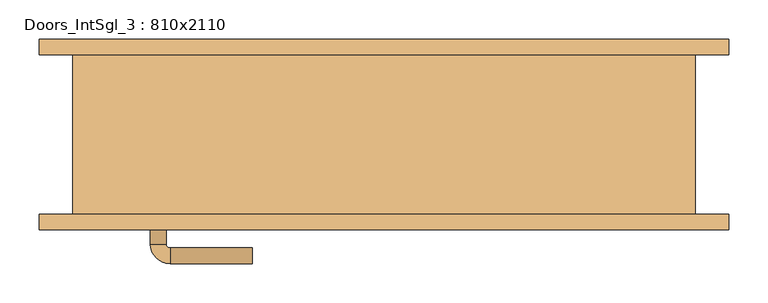
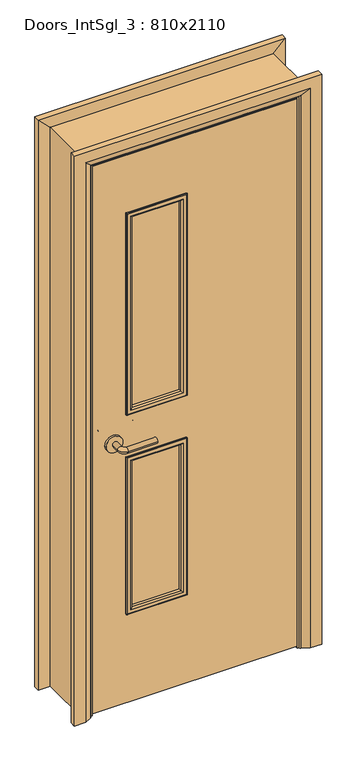
"""IFC4 building model written with IfcOpenShell, lengths in millimetres: door geometry, Doors_IntSgl_3 : 810x2110."""

from ifc_helpers import new_model, si_unit, point, frame, frame_2d, origin, place, context, project, spatial, polyline, circle_curve, ellipse_curve, trimmed, segment, composite_curve, outline, extrude, faceted_brep, source, transform, mapped, element, save
from ifc_brep_helpers import plane_surface, cylinder_surface, revolved_surface, advanced_brep


def doors_intsgl_3_810x2110_fc3e9706(model_context):
    return source(origin(), model_context, "Body", "SolidModel", [
        advanced_brep(
        [(-298.0, -55.6, 1000.0), (-278.0, -55.6, 1000.0), (-298.0, -25.6, 1000.0), (-278.0, -25.6, 1000.0), (-273.0, -20.6, 1000.0), (-273.0, -0.6, 1000.0), (-168.0, -0.6, 1000.0), (-168.0, -20.6, 1000.0)],
        [
            (0, 1, circle_curve(frame((-288.0, -55.6, 1000.0), z_axis=(0.0, -1.0, 0.0), x_axis=(1.0, 0.0, 0.0)), 10.0)),
            (1, 0, circle_curve(frame((-288.0, -55.6, 1000.0), z_axis=(0.0, -1.0, 0.0), x_axis=(1.0, 0.0, 0.0)), 10.0)),
            (0, 2),
            (2, 3, circle_curve(frame((-288.0, -25.6, 1000.0), z_axis=(0.0, -1.0, 0.0), x_axis=(1.0, 0.0, 0.0)), 10.0)),
            (3, 1),
            (3, 2, circle_curve(frame((-288.0, -25.6, 1000.0), z_axis=(0.0, -1.0, 0.0), x_axis=(1.0, 0.0, 0.0)), 10.0)),
            (4, 3, circle_curve(frame((-273.0, -25.6, 1000.0), z_axis=(0.0, 0.0, 1.0), x_axis=(-1.0, 0.0, 0.0)), 5.0)),
            (2, 5, circle_curve(frame((-273.0, -25.6, 1000.0), z_axis=(0.0, 0.0, -1.0), x_axis=(-1.0, 0.0, 0.0)), 25.0)),
            (5, 4, circle_curve(frame((-273.0, -10.6, 1000.0), z_axis=(-1.0, 0.0, 0.0), x_axis=(0.0, -1.0, 0.0)), 10.0)),
            (4, 5, circle_curve(frame((-273.0, -10.6, 1000.0), z_axis=(-1.0, 0.0, 0.0), x_axis=(0.0, -1.0, 0.0)), 10.0)),
            (6, 7, circle_curve(frame((-168.0, -10.6, 1000.0), z_axis=(1.0, 0.0, 0.0), x_axis=(0.0, -1.0, 0.0)), 10.0)),
            (7, 6, circle_curve(frame((-168.0, -10.6, 1000.0), z_axis=(1.0, 0.0, 0.0), x_axis=(0.0, -1.0, 0.0)), 10.0)),
            (5, 6),
            (7, 4),
        ],
        [
            plane_surface(frame((-288.0, -55.6, 1000.0), z_axis=(0.0, -1.0, 0.0), x_axis=(0.0, 0.0, 1.0))),
            cylinder_surface(frame((-288.0, -55.6, 1000.0), z_axis=(0.0, -1.0, 0.0), x_axis=(1.0, 0.0, 0.0)), 10.0),
            revolved_surface(trimmed(ellipse_curve(frame((-288.0, -25.6, 1000.0), z_axis=(0.0, -1.0, 0.0), x_axis=(1.0, 0.0, 0.0)), 10.0, 10.0), [point((-298.0, -25.6, 1000.0))], [point((-278.0, -25.6, 1000.0))], True, "CARTESIAN"), (-273.0, -25.6, 1000.0), (0.0, 0.0, -1.0)),
            revolved_surface(trimmed(ellipse_curve(frame((-288.0, -25.6, 1000.0), z_axis=(0.0, -1.0, 0.0), x_axis=(1.0, 0.0, 0.0)), 10.0, 10.0), [point((-278.0, -25.6, 1000.0))], [point((-298.0, -25.6, 1000.0))], True, "CARTESIAN"), (-273.0, -25.6, 1000.0), (0.0, 0.0, -1.0)),
            plane_surface(frame((-168.0, -10.6, 1000.0), z_axis=(1.0, 0.0, 0.0), x_axis=(0.0, 0.0, 1.0))),
            cylinder_surface(frame((-273.0, -10.6, 1000.0), z_axis=(-1.0, 0.0, 0.0), x_axis=(0.0, -1.0, 0.0)), 10.0),
        ],
        [
            (0, [[1, 2]]),
            (1, [[-1, 3, 4, 5]]),
            (1, [[-2, -5, 6, -3]]),
            (2, [[7, -4, 8, 9]]),
            (3, [[-8, -6, -7, 10]]),
            (4, [[11, 12]]),
            (5, [[-9, 13, -12, 14]]),
            (5, [[-10, -14, -11, -13]]),
        ],
    ),
        extrude(outline(composite_curve([segment(trimmed(circle_curve(frame_2d((1000.0, -290.5)), 30.0), [point((1000.0, -320.5))], [point((1000.0, -260.5))], False, "CARTESIAN"), True, "CONTINUOUS"), segment(trimmed(circle_curve(frame_2d((1000.0, -290.5)), 30.0), [point((1000.0, -260.5))], [point((1000.0, -320.5))], False, "CARTESIAN"), True, "CONTINUOUS")], self_intersect=False)), frame((0.0, -63.6, 0.0), z_axis=(0.0, 1.0, 0.0), x_axis=(0.0, 0.0, 1.0)), (0.0, 0.0, 1.0), 8.0),
        advanced_brep(
        [(-298.0, -109.6, 1000.0), (-278.0, -109.6, 1000.0), (-278.0, -139.6, 1000.0), (-298.0, -139.6, 1000.0), (-273.0, -144.6, 1000.0), (-273.0, -164.6, 1000.0), (-168.0, -164.6, 1000.0), (-168.0, -144.6, 1000.0)],
        [
            (0, 1, circle_curve(frame((-288.0, -109.6, 1000.0), z_axis=(0.0, 1.0, 0.0), x_axis=(1.0, 0.0, 0.0)), 10.0)),
            (1, 0, circle_curve(frame((-288.0, -109.6, 1000.0), z_axis=(0.0, 1.0, 0.0), x_axis=(1.0, 0.0, 0.0)), 10.0)),
            (1, 2),
            (2, 3, circle_curve(frame((-288.0, -139.6, 1000.0), z_axis=(0.0, 1.0, 0.0), x_axis=(1.0, 0.0, 0.0)), 10.0)),
            (3, 0),
            (3, 2, circle_curve(frame((-288.0, -139.6, 1000.0), z_axis=(0.0, 1.0, 0.0), x_axis=(1.0, 0.0, 0.0)), 10.0)),
            (4, 5, circle_curve(frame((-273.0, -154.6, 1000.0), z_axis=(-1.0, 0.0, 0.0), x_axis=(0.0, 1.0, 0.0)), 10.0)),
            (5, 3, circle_curve(frame((-273.0, -139.6, 1000.0), z_axis=(0.0, 0.0, -1.0), x_axis=(-1.0, 0.0, 0.0)), 25.0)),
            (2, 4, circle_curve(frame((-273.0, -139.6, 1000.0), z_axis=(0.0, 0.0, 1.0), x_axis=(-1.0, 0.0, 0.0)), 5.0)),
            (5, 4, circle_curve(frame((-273.0, -154.6, 1000.0), z_axis=(-1.0, 0.0, 0.0), x_axis=(0.0, 1.0, 0.0)), 10.0)),
            (6, 7, circle_curve(frame((-168.0, -154.6, 1000.0), z_axis=(1.0, 0.0, 0.0), x_axis=(0.0, 1.0, 0.0)), 10.0)),
            (7, 6, circle_curve(frame((-168.0, -154.6, 1000.0), z_axis=(1.0, 0.0, 0.0), x_axis=(0.0, 1.0, 0.0)), 10.0)),
            (4, 7),
            (6, 5),
        ],
        [
            plane_surface(frame((-288.0, -109.6, 1000.0), z_axis=(0.0, 1.0, 0.0), x_axis=(0.0, 0.0, 1.0))),
            cylinder_surface(frame((-288.0, -109.6, 1000.0), z_axis=(0.0, 1.0, 0.0), x_axis=(1.0, 0.0, 0.0)), 10.0),
            revolved_surface(trimmed(ellipse_curve(frame((-288.0, -139.6, 1000.0), z_axis=(0.0, -1.0, 0.0), x_axis=(1.0, 0.0, 0.0)), 10.0, 10.0), [point((-298.0, -139.6, 1000.0))], [point((-278.0, -139.6, 1000.0))], True, "CARTESIAN"), (-273.0, -139.6, 1000.0), (0.0, 0.0, -1.0)),
            revolved_surface(trimmed(ellipse_curve(frame((-288.0, -139.6, 1000.0), z_axis=(0.0, -1.0, 0.0), x_axis=(1.0, 0.0, 0.0)), 10.0, 10.0), [point((-278.0, -139.6, 1000.0))], [point((-298.0, -139.6, 1000.0))], True, "CARTESIAN"), (-273.0, -139.6, 1000.0), (0.0, 0.0, -1.0)),
            plane_surface(frame((-168.0, -154.6, 1000.0), z_axis=(1.0, 0.0, 0.0), x_axis=(0.0, 0.0, 1.0))),
            cylinder_surface(frame((-273.0, -154.6, 1000.0), z_axis=(-1.0, 0.0, 0.0), x_axis=(0.0, 1.0, 0.0)), 10.0),
        ],
        [
            (0, [[1, 2]]),
            (1, [[3, 4, 5, -2]]),
            (1, [[-5, 6, -3, -1]]),
            (2, [[7, 8, -4, 9]]),
            (3, [[10, -9, -6, -8]]),
            (4, [[11, 12]]),
            (5, [[13, -11, 14, -7]]),
            (5, [[-14, -12, -13, -10]]),
        ],
    ),
        extrude(outline(composite_curve([segment(trimmed(circle_curve(frame_2d((1000.0, -290.5)), 30.0), [point((1000.0, -320.5))], [point((1000.0, -260.5))], False, "CARTESIAN"), True, "CONTINUOUS"), segment(trimmed(circle_curve(frame_2d((1000.0, -290.5)), 30.0), [point((1000.0, -260.5))], [point((1000.0, -320.5))], False, "CARTESIAN"), True, "CONTINUOUS")], self_intersect=False)), frame((0.0, -109.6, 0.0), z_axis=(0.0, 1.0, 0.0), x_axis=(0.0, 0.0, 1.0)), (0.0, 0.0, 1.0), 8.0),
        extrude(outline(polyline([(2068.0, -363.0), (8.0, -363.0), (8.0, 363.0), (2068.0, 363.0), (2068.0, -363.0)]), holes=[polyline([(1843.0, -38.0), (1100.0, -38.0), (1100.0, -238.0), (1843.0, -238.0), (1843.0, -38.0)]), polyline([(925.0, -238.0), (925.0, -38.0), (350.0, -38.0), (350.0, -238.0), (925.0, -238.0)])]), frame((0.0, -101.6, 0.0), z_axis=(0.0, 1.0, 0.0), x_axis=(0.0, 0.0, 1.0)), (0.0, 0.0, 1.0), 38.0),
        faceted_brep([(-365.0, -101.6, 0.0), (-397.0, -101.6, 0.0), (-397.0, 101.6, 0.0), (-365.0, 101.6, 0.0), (-365.0, 101.6, 2070.0), (-365.0, -101.6, 2070.0), (-397.0, 101.6, 2102.0), (-397.0, -101.6, 2102.0), (365.0, -101.6, 0.0), (365.0, 101.6, 0.0), (397.0, 101.6, 0.0), (397.0, -101.6, 0.0), (365.0, -101.6, 2070.0), (397.0, -101.6, 2102.0), (397.0, 101.6, 2102.0), (365.0, 101.6, 2070.0)], [[[0, 1, 2, 3]], [[3, 4, 5, 0]], [[2, 6, 4, 3]], [[1, 7, 6, 2]], [[0, 5, 7, 1]], [[8, 9, 10, 11]], [[12, 8, 11, 13]], [[13, 11, 10, 14]], [[14, 10, 9, 15]], [[15, 9, 8, 12]], [[4, 15, 12, 5]], [[6, 14, 15, 4]], [[7, 13, 14, 6]], [[5, 12, 13, 7]]]),
        advanced_brep(
        [(-440.0, 121.6, 0.0), (-400.0, 121.6, 0.0), (-374.0, 107.6, 0.0), (-370.0, 101.6, 0.0), (-440.0, 101.6, 0.0), (-440.0, 101.6, 2145.0), (-440.0, 121.6, 2145.0), (-370.0, 101.6, 2075.0), (-374.0, 107.6, 2079.0), (-400.0, 121.6, 2105.0), (440.0, 121.6, 0.0), (440.0, 101.6, 0.0), (370.0, 101.6, 0.0), (374.0, 107.6, 0.0), (400.0, 121.6, 0.0), (440.0, 121.6, 2145.0), (400.0, 121.6, 2105.0), (374.0, 107.6, 2079.0), (370.0, 101.6, 2075.0), (440.0, 101.6, 2145.0)],
        [
            (0, 1),
            (1, 2),
            (2, 3, circle_curve(frame((-378.0, 100.6, 0.0), z_axis=(0.0, 0.0, -1.0), x_axis=(-1.0, 0.0, 0.0)), 8.0622577)),
            (3, 4),
            (4, 0),
            (4, 5),
            (5, 6),
            (6, 0),
            (3, 7),
            (7, 5),
            (2, 8),
            (8, 7, ellipse_curve(frame((-378.0, 100.6, 2083.0), z_axis=(-0.7071067811865475, 0.0, -0.7071067811865475), x_axis=(0.7071067811865474, 0.0, -0.7071067811865476)), 11.4017543, 8.0622577)),
            (1, 9),
            (9, 8),
            (6, 9),
            (10, 11),
            (11, 12),
            (12, 13, circle_curve(frame((378.0, 100.6, 0.0), z_axis=(0.0, 0.0, -1.0), x_axis=(1.0, 0.0, 0.0)), 8.0622577)),
            (13, 14),
            (14, 10),
            (15, 10),
            (14, 16),
            (16, 15),
            (13, 17),
            (17, 16),
            (12, 18),
            (18, 17, ellipse_curve(frame((378.0, 100.6, 2083.0), z_axis=(0.7071067811865475, 0.0, -0.7071067811865475), x_axis=(0.7071067811865474, 0.0, 0.7071067811865476)), 11.4017543, 8.0622577)),
            (11, 19),
            (19, 18),
            (15, 19),
            (5, 19),
            (15, 6),
            (7, 18),
            (8, 17),
            (9, 16),
        ],
        [
            plane_surface(frame((-370.0, 174.4010989, 0.0), z_axis=(0.0, 0.0, -1.0), x_axis=(1.0, 0.0, 0.0))),
            plane_surface(frame((-440.0, 121.6, 0.0), z_axis=(-1.0, 0.0, 0.0), x_axis=(0.0, 0.0, 1.0))),
            plane_surface(frame((-440.0, 101.6, 0.0), z_axis=(0.0, -1.0, 0.0), x_axis=(0.0, 0.0, 1.0))),
            cylinder_surface(frame((-378.0, 100.6, 0.0), z_axis=(0.0, 0.0, -1.0), x_axis=(-1.0, 0.0, 0.0)), 8.0622577),
            plane_surface(frame((-374.0, 107.6, 0.0), z_axis=(0.4740998230350183, 0.8804710999221749, 0.0), x_axis=(0.0, 0.0, 1.0))),
            plane_surface(frame((-400.0, 121.6, 0.0), z_axis=(0.0, 1.0, 0.0), x_axis=(0.0, 0.0, 1.0))),
            plane_surface(frame((370.0, 174.4010989, 0.0), z_axis=(0.0, 0.0, -1.0), x_axis=(-1.0, 0.0, 0.0))),
            plane_surface(frame((400.0, 121.6, 2105.0), z_axis=(0.0, 1.0, 0.0), x_axis=(0.0, 0.0, -1.0))),
            plane_surface(frame((374.0, 107.6, 2079.0), z_axis=(-0.4740998230350183, 0.8804710999221749, 0.0), x_axis=(0.0, 0.0, -1.0))),
            cylinder_surface(frame((378.0, 100.6, 2075.0), z_axis=(0.0, 0.0, 1.0), x_axis=(1.0, 0.0, 0.0)), 8.0622577),
            plane_surface(frame((440.0, 101.6, 2145.0), z_axis=(0.0, -1.0, 0.0), x_axis=(0.0, 0.0, -1.0))),
            plane_surface(frame((440.0, 121.6, 2145.0), z_axis=(1.0, 0.0, 0.0), x_axis=(0.0, 0.0, -1.0))),
            plane_surface(frame((-440.0, 121.6, 2145.0), z_axis=(0.0, 0.0, 1.0), x_axis=(1.0, 0.0, 0.0))),
            plane_surface(frame((-440.0, 101.6, 2145.0), z_axis=(0.0, -1.0, 0.0), x_axis=(1.0, 0.0, 0.0))),
            cylinder_surface(frame((-370.0, 100.6, 2083.0), z_axis=(-1.0, 0.0, 0.0), x_axis=(0.0, 0.0, 1.0)), 8.0622577),
            plane_surface(frame((-374.0, 107.6, 2079.0), z_axis=(0.0, 0.8804710999221749, -0.4740998230350183), x_axis=(1.0, 0.0, 0.0))),
            plane_surface(frame((-400.0, 121.6, 2105.0), z_axis=(0.0, 1.0, 0.0), x_axis=(1.0, 0.0, 0.0))),
        ],
        [
            (0, [[1, 2, 3, 4, 5]]),
            (1, [[6, 7, 8, -5]]),
            (2, [[9, 10, -6, -4]]),
            (3, [[11, 12, -9, -3]]),
            (4, [[13, 14, -11, -2]]),
            (5, [[-8, 15, -13, -1]]),
            (6, [[16, 17, 18, 19, 20]]),
            (7, [[21, -20, 22, 23]]),
            (8, [[-22, -19, 24, 25]]),
            (9, [[-24, -18, 26, 27]]),
            (10, [[-26, -17, 28, 29]]),
            (11, [[-28, -16, -21, 30]]),
            (12, [[31, -30, 32, -7]]),
            (13, [[33, -29, -31, -10]]),
            (14, [[34, -27, -33, -12]]),
            (15, [[35, -25, -34, -14]]),
            (16, [[-32, -23, -35, -15]]),
        ],
    ),
        extrude(outline(polyline([(0.0, -346.0), (2051.0, -346.0), (2051.0, 346.0), (0.0, 346.0), (0.0, 365.0), (2070.0, 365.0), (2070.0, -365.0), (0.0, -365.0), (0.0, -346.0)])), frame((0.0, -61.6, 0.0), z_axis=(0.0, 1.0, 0.0), x_axis=(0.0, 0.0, 1.0)), (0.0, 0.0, 1.0), 32.0),
        advanced_brep(
        [(440.0, -121.6, 0.0), (400.0, -121.6, 0.0), (374.0, -107.6, 0.0), (370.0, -101.6, 0.0), (440.0, -101.6, 0.0), (440.0, -101.6, 2145.0), (440.0, -121.6, 2145.0), (370.0, -101.6, 2075.0), (-370.0, -101.6, 2075.0), (-370.0, -101.6, 0.0), (-440.0, -101.6, 0.0), (-440.0, -101.6, 2145.0), (374.0, -107.6, 2079.0), (400.0, -121.6, 2105.0), (-440.0, -121.6, 2145.0), (-440.0, -121.6, 0.0), (-400.0, -121.6, 0.0), (-400.0, -121.6, 2105.0), (-374.0, -107.6, 0.0), (-374.0, -107.6, 2079.0)],
        [
            (0, 1),
            (1, 2),
            (2, 3, circle_curve(frame((378.0, -100.6, 0.0), z_axis=(0.0, 0.0, -1.0), x_axis=(1.0, 0.0, 0.0)), 8.0622577)),
            (3, 4),
            (4, 0),
            (4, 5),
            (5, 6),
            (6, 0),
            (3, 7),
            (7, 8),
            (8, 9),
            (9, 10),
            (10, 11),
            (11, 5),
            (2, 12),
            (12, 7, ellipse_curve(frame((378.0, -100.6, 2083.0), z_axis=(0.7071067811865475, 0.0, -0.7071067811865475), x_axis=(-0.7071067811865474, 0.0, -0.7071067811865476)), 11.4017543, 8.0622577)),
            (1, 13),
            (13, 12),
            (6, 14),
            (14, 15),
            (15, 16),
            (16, 17),
            (17, 13),
            (10, 15),
            (14, 11),
            (9, 18, circle_curve(frame((-378.0, -100.6, 0.0), z_axis=(0.0, 0.0, -1.0), x_axis=(-1.0, 0.0, 0.0)), 8.0622577)),
            (18, 16),
            (19, 18),
            (8, 19, ellipse_curve(frame((-378.0, -100.6, 2083.0), z_axis=(-0.7071067811865475, 0.0, -0.7071067811865475), x_axis=(-0.7071067811865474, 0.0, 0.7071067811865476)), 11.4017543, 8.0622577)),
            (19, 17),
            (12, 19),
        ],
        [
            plane_surface(frame((370.0, -101.6, 0.0), z_axis=(0.0, 0.0, -1.0), x_axis=(0.0, 1.0, 0.0))),
            plane_surface(frame((440.0, -121.6, 0.0), z_axis=(1.0, 0.0, 0.0), x_axis=(0.0, 0.0, 1.0))),
            plane_surface(frame((440.0, -101.6, 0.0), z_axis=(0.0, 1.0, 0.0), x_axis=(0.0, 0.0, 1.0))),
            cylinder_surface(frame((378.0, -100.6, 0.0), z_axis=(0.0, 0.0, -1.0), x_axis=(1.0, 0.0, 0.0)), 8.0622577),
            plane_surface(frame((374.0, -107.6, 0.0), z_axis=(-0.4740998230350126, -0.8804710999221779, 0.0), x_axis=(0.0, 0.0, 1.0))),
            plane_surface(frame((400.0, -121.6, 0.0), z_axis=(0.0, -1.0, 0.0), x_axis=(0.0, 0.0, 1.0))),
            plane_surface(frame((-440.0, -121.6, 2145.0), z_axis=(-1.0, 0.0, 0.0), x_axis=(0.0, 0.0, -1.0))),
            plane_surface(frame((-370.0, -101.6, 0.0), z_axis=(0.0, 0.0, -1.0), x_axis=(0.0, 1.0, 0.0))),
            cylinder_surface(frame((-378.0, -100.6, 2075.0), z_axis=(0.0, 0.0, 1.0), x_axis=(-1.0, 0.0, 0.0)), 8.0622577),
            plane_surface(frame((-374.0, -107.6, 2079.0), z_axis=(0.4740998230350183, -0.8804710999221749, 0.0), x_axis=(0.0, 0.0, -1.0))),
            plane_surface(frame((440.0, -121.6, 2145.0), z_axis=(0.0, 0.0, 1.0), x_axis=(-1.0, 0.0, 0.0))),
            cylinder_surface(frame((370.0, -100.6, 2083.0), z_axis=(1.0, 0.0, 0.0), x_axis=(0.0, 0.0, 1.0)), 8.0622577),
            plane_surface(frame((374.0, -107.6, 2079.0), z_axis=(0.0, -0.8804710999221763, -0.4740998230350154), x_axis=(-1.0, 0.0, 0.0))),
        ],
        [
            (0, [[1, 2, 3, 4, 5]]),
            (1, [[6, 7, 8, -5]]),
            (2, [[9, 10, 11, 12, 13, 14, -6, -4]]),
            (3, [[15, 16, -9, -3]]),
            (4, [[17, 18, -15, -2]]),
            (5, [[-8, 19, 20, 21, 22, 23, -17, -1]]),
            (6, [[-13, 24, -20, 25]]),
            (7, [[-24, -12, 26, 27, -21]]),
            (8, [[28, -26, -11, 29]]),
            (9, [[-22, -27, -28, 30]]),
            (10, [[-14, -25, -19, -7]]),
            (11, [[31, -29, -10, -16]]),
            (12, [[-23, -30, -31, -18]]),
        ],
    ),
        advanced_brep(
        [(-30.0, -105.6, 1851.0), (-30.0, -105.6, 1092.0), (-30.0, -101.6, 1092.0), (-30.0, -101.6, 1851.0), (-32.0, -107.6, 1849.0), (-32.0, -107.6, 1094.0), (-50.0, -102.6, 1831.0), (-50.0, -102.6, 1112.0), (-45.0, -107.6, 1107.0), (-45.0, -107.6, 1836.0), (-50.0, -91.6, 1831.0), (-50.0, -91.6, 1112.0), (-38.0, -101.6, 1843.0), (-38.0, -101.6, 1100.0), (-38.0, -91.6, 1100.0), (-38.0, -91.6, 1843.0), (-246.0, -105.6, 1092.0), (-246.0, -101.6, 1092.0), (-244.0, -107.6, 1094.0), (-226.0, -102.6, 1112.0), (-231.0, -107.6, 1107.0), (-226.0, -91.6, 1112.0), (-238.0, -101.6, 1100.0), (-238.0, -91.6, 1100.0), (-246.0, -105.6, 1851.0), (-246.0, -101.6, 1851.0), (-244.0, -107.6, 1849.0), (-226.0, -102.6, 1831.0), (-231.0, -107.6, 1836.0), (-226.0, -91.6, 1831.0), (-238.0, -101.6, 1843.0), (-238.0, -91.6, 1843.0)],
        [
            (0, 1),
            (1, 2),
            (2, 3),
            (3, 0),
            (4, 5),
            (5, 1, ellipse_curve(frame((-32.0, -105.6, 1094.0), z_axis=(0.7071067811865475, 0.0, 0.7071067811865475), x_axis=(-0.7071067811865474, 0.0, 0.7071067811865476)), 2.8284271, 2.0)),
            (0, 4, ellipse_curve(frame((-32.0, -105.6, 1849.0), z_axis=(0.7071067811865475, 0.0, -0.7071067811865475), x_axis=(0.7071067811865474, 0.0, 0.7071067811865476)), 2.8284271, 2.0)),
            (6, 7),
            (7, 8, ellipse_curve(frame((-45.0, -102.6, 1107.0), z_axis=(0.7071067811865475, 0.0, 0.7071067811865475), x_axis=(-0.7071067811865474, 0.0, 0.7071067811865476)), 7.0710678, 5.0)),
            (8, 9),
            (9, 6, ellipse_curve(frame((-45.0, -102.6, 1836.0), z_axis=(0.7071067811865475, 0.0, -0.7071067811865475), x_axis=(0.7071067811865474, 0.0, 0.7071067811865476)), 7.0710678, 5.0)),
            (10, 11),
            (11, 7),
            (6, 10),
            (12, 13),
            (13, 14),
            (14, 15),
            (15, 12),
            (1, 16),
            (16, 17),
            (17, 2),
            (5, 18),
            (18, 16, ellipse_curve(frame((-244.0, -105.6, 1094.0), z_axis=(0.7071067811865475, 0.0, -0.7071067811865475), x_axis=(0.7071067811865476, 0.0, 0.7071067811865474)), 2.8284271, 2.0)),
            (7, 19),
            (19, 20, ellipse_curve(frame((-231.0, -102.6, 1107.0), z_axis=(0.7071067811865475, 0.0, -0.7071067811865475), x_axis=(0.7071067811865476, 0.0, 0.7071067811865474)), 7.0710678, 5.0)),
            (20, 8),
            (11, 21),
            (21, 19),
            (13, 22),
            (22, 23),
            (23, 14),
            (16, 24),
            (24, 25),
            (25, 17),
            (18, 26),
            (26, 24, ellipse_curve(frame((-244.0, -105.6, 1849.0), z_axis=(-0.7071067811865475, 0.0, -0.7071067811865475), x_axis=(0.7071067811865474, 0.0, -0.7071067811865476)), 2.8284271, 2.0)),
            (19, 27),
            (27, 28, ellipse_curve(frame((-231.0, -102.6, 1836.0), z_axis=(-0.7071067811865475, 0.0, -0.7071067811865475), x_axis=(0.7071067811865474, 0.0, -0.7071067811865476)), 7.0710678, 5.0)),
            (28, 20),
            (21, 29),
            (29, 27),
            (22, 30),
            (30, 31),
            (31, 23),
            (24, 0),
            (3, 25),
            (26, 4),
            (28, 9),
            (27, 6),
            (29, 10),
            (31, 15),
            (30, 12),
        ],
        [
            plane_surface(frame((-30.0, -101.6, 1851.0), z_axis=(1.0, 0.0, 0.0), x_axis=(0.0, 0.0, -1.0))),
            cylinder_surface(frame((-32.0, -105.6, 1843.0), z_axis=(0.0, 0.0, 1.0), x_axis=(1.0, 0.0, 0.0)), 2.0),
            cylinder_surface(frame((-45.0, -102.6, 1843.0), z_axis=(0.0, 0.0, 1.0), x_axis=(1.0, 0.0, 0.0)), 5.0),
            plane_surface(frame((-50.0, -102.6, 1831.0), z_axis=(-1.0, 0.0, 0.0), x_axis=(0.0, 0.0, -1.0))),
            plane_surface(frame((-38.0, -91.6, 1843.0), z_axis=(1.0, 0.0, 0.0), x_axis=(0.0, 0.0, -1.0))),
            plane_surface(frame((-30.0, -101.6, 1092.0), z_axis=(0.0, 0.0, -1.0), x_axis=(-1.0, 0.0, 0.0))),
            cylinder_surface(frame((-38.0, -105.6, 1094.0), z_axis=(1.0, 0.0, 0.0), x_axis=(0.0, 0.0, -1.0)), 2.0),
            cylinder_surface(frame((-38.0, -102.6, 1107.0), z_axis=(1.0, 0.0, 0.0), x_axis=(0.0, 0.0, -1.0)), 5.0),
            plane_surface(frame((-50.0, -102.6, 1112.0), z_axis=(0.0, 0.0, 1.0), x_axis=(-1.0, 0.0, 0.0))),
            plane_surface(frame((-38.0, -91.6, 1100.0), z_axis=(0.0, 0.0, -1.0), x_axis=(-1.0, 0.0, 0.0))),
            plane_surface(frame((-246.0, -101.6, 1092.0), z_axis=(-1.0, 0.0, 0.0), x_axis=(0.0, 0.0, 1.0))),
            cylinder_surface(frame((-244.0, -105.6, 1100.0), z_axis=(0.0, 0.0, -1.0), x_axis=(-1.0, 0.0, 0.0)), 2.0),
            cylinder_surface(frame((-231.0, -102.6, 1100.0), z_axis=(0.0, 0.0, -1.0), x_axis=(-1.0, 0.0, 0.0)), 5.0),
            plane_surface(frame((-226.0, -102.6, 1112.0), z_axis=(1.0, 0.0, 0.0), x_axis=(0.0, 0.0, 1.0))),
            plane_surface(frame((-238.0, -91.6, 1100.0), z_axis=(-1.0, 0.0, 0.0), x_axis=(0.0, 0.0, 1.0))),
            plane_surface(frame((-246.0, -101.6, 1851.0), z_axis=(0.0, 0.0, 1.0), x_axis=(1.0, 0.0, 0.0))),
            cylinder_surface(frame((-238.0, -105.6, 1849.0), z_axis=(-1.0, 0.0, 0.0), x_axis=(0.0, 0.0, 1.0)), 2.0),
            plane_surface(frame((-244.0, -107.6, 1849.0), z_axis=(0.0, -1.0, 0.0), x_axis=(1.0, 0.0, 0.0))),
            cylinder_surface(frame((-238.0, -102.6, 1836.0), z_axis=(-1.0, 0.0, 0.0), x_axis=(0.0, 0.0, 1.0)), 5.0),
            plane_surface(frame((-226.0, -102.6, 1831.0), z_axis=(0.0, 0.0, -1.0), x_axis=(1.0, 0.0, 0.0))),
            plane_surface(frame((-226.0, -91.6, 1831.0), z_axis=(0.0, 1.0, 0.0), x_axis=(1.0, 0.0, 0.0))),
            plane_surface(frame((-238.0, -91.6, 1843.0), z_axis=(0.0, 0.0, 1.0), x_axis=(1.0, 0.0, 0.0))),
            plane_surface(frame((-238.0, -101.6, 1843.0), z_axis=(0.0, 1.0, 0.0), x_axis=(1.0, 0.0, 0.0))),
        ],
        [
            (0, [[1, 2, 3, 4]]),
            (1, [[5, 6, -1, 7]]),
            (2, [[8, 9, 10, 11]]),
            (3, [[12, 13, -8, 14]]),
            (4, [[15, 16, 17, 18]]),
            (5, [[19, 20, 21, -2]]),
            (6, [[22, 23, -19, -6]]),
            (7, [[24, 25, 26, -9]]),
            (8, [[27, 28, -24, -13]]),
            (9, [[29, 30, 31, -16]]),
            (10, [[32, 33, 34, -20]]),
            (11, [[35, 36, -32, -23]]),
            (12, [[37, 38, 39, -25]]),
            (13, [[40, 41, -37, -28]]),
            (14, [[42, 43, 44, -30]]),
            (15, [[45, -4, 46, -33]]),
            (16, [[47, -7, -45, -36]]),
            (17, [[-5, -47, -35, -22], [-10, -26, -39, 48]]),
            (18, [[49, -11, -48, -38]]),
            (19, [[50, -14, -49, -41]]),
            (20, [[-17, -31, -44, 51], [-12, -50, -40, -27]]),
            (21, [[52, -18, -51, -43]]),
            (22, [[-3, -21, -34, -46], [-15, -52, -42, -29]]),
        ],
    ),
        advanced_brep(
        [(-38.0, -73.6, 1843.0), (-38.0, -73.6, 1100.0), (-38.0, -63.6, 1100.0), (-38.0, -63.6, 1843.0), (-50.0, -62.6, 1831.0), (-50.0, -62.6, 1112.0), (-50.0, -73.6, 1112.0), (-50.0, -73.6, 1831.0), (-45.0, -57.6, 1836.0), (-45.0, -57.6, 1107.0), (-30.0, -59.6, 1851.0), (-30.0, -59.6, 1092.0), (-32.0, -57.6, 1094.0), (-32.0, -57.6, 1849.0), (-30.0, -63.6, 1851.0), (-30.0, -63.6, 1092.0), (-238.0, -73.6, 1100.0), (-238.0, -63.6, 1100.0), (-226.0, -62.6, 1112.0), (-226.0, -73.6, 1112.0), (-231.0, -57.6, 1107.0), (-246.0, -59.6, 1092.0), (-244.0, -57.6, 1094.0), (-246.0, -63.6, 1092.0), (-238.0, -73.6, 1843.0), (-238.0, -63.6, 1843.0), (-226.0, -62.6, 1831.0), (-226.0, -73.6, 1831.0), (-231.0, -57.6, 1836.0), (-246.0, -59.6, 1851.0), (-244.0, -57.6, 1849.0), (-246.0, -63.6, 1851.0)],
        [
            (0, 1),
            (1, 2),
            (2, 3),
            (3, 0),
            (4, 5),
            (5, 6),
            (6, 7),
            (7, 4),
            (8, 9),
            (9, 5, ellipse_curve(frame((-45.0, -62.6, 1107.0), z_axis=(0.7071067811865475, 0.0, 0.7071067811865475), x_axis=(-0.7071067811865474, 0.0, 0.7071067811865476)), 7.0710678, 5.0)),
            (4, 8, ellipse_curve(frame((-45.0, -62.6, 1836.0), z_axis=(0.7071067811865475, 0.0, -0.7071067811865475), x_axis=(0.7071067811865474, 0.0, 0.7071067811865476)), 7.0710678, 5.0)),
            (10, 11),
            (11, 12, ellipse_curve(frame((-32.0, -59.6, 1094.0), z_axis=(0.7071067811865475, 0.0, 0.7071067811865475), x_axis=(-0.7071067811865474, 0.0, 0.7071067811865476)), 2.8284271, 2.0)),
            (12, 13),
            (13, 10, ellipse_curve(frame((-32.0, -59.6, 1849.0), z_axis=(0.7071067811865475, 0.0, -0.7071067811865475), x_axis=(0.7071067811865474, 0.0, 0.7071067811865476)), 2.8284271, 2.0)),
            (14, 15),
            (15, 11),
            (10, 14),
            (1, 16),
            (16, 17),
            (17, 2),
            (5, 18),
            (18, 19),
            (19, 6),
            (9, 20),
            (20, 18, ellipse_curve(frame((-231.0, -62.6, 1107.0), z_axis=(0.7071067811865475, 0.0, -0.7071067811865475), x_axis=(0.7071067811865476, 0.0, 0.7071067811865474)), 7.0710678, 5.0)),
            (11, 21),
            (21, 22, ellipse_curve(frame((-244.0, -59.6, 1094.0), z_axis=(0.7071067811865475, 0.0, -0.7071067811865475), x_axis=(0.7071067811865476, 0.0, 0.7071067811865474)), 2.8284271, 2.0)),
            (22, 12),
            (15, 23),
            (23, 21),
            (16, 24),
            (24, 25),
            (25, 17),
            (18, 26),
            (26, 27),
            (27, 19),
            (20, 28),
            (28, 26, ellipse_curve(frame((-231.0, -62.6, 1836.0), z_axis=(-0.7071067811865475, 0.0, -0.7071067811865475), x_axis=(0.7071067811865474, 0.0, -0.7071067811865476)), 7.0710678, 5.0)),
            (21, 29),
            (29, 30, ellipse_curve(frame((-244.0, -59.6, 1849.0), z_axis=(-0.7071067811865475, 0.0, -0.7071067811865475), x_axis=(0.7071067811865474, 0.0, -0.7071067811865476)), 2.8284271, 2.0)),
            (30, 22),
            (23, 31),
            (31, 29),
            (14, 31),
            (25, 3),
            (24, 0),
            (27, 7),
            (26, 4),
            (28, 8),
            (30, 13),
            (29, 10),
        ],
        [
            plane_surface(frame((-38.0, -63.6, 1843.0), z_axis=(1.0, 0.0, 0.0), x_axis=(0.0, 0.0, -1.0))),
            plane_surface(frame((-50.0, -73.6, 1831.0), z_axis=(-1.0, 0.0, 0.0), x_axis=(0.0, 0.0, -1.0))),
            cylinder_surface(frame((-45.0, -62.6, 1843.0), z_axis=(0.0, 0.0, 1.0), x_axis=(1.0, 0.0, 0.0)), 5.0),
            cylinder_surface(frame((-32.0, -59.6, 1843.0), z_axis=(0.0, 0.0, 1.0), x_axis=(1.0, 0.0, 0.0)), 2.0),
            plane_surface(frame((-30.0, -59.6, 1851.0), z_axis=(1.0, 0.0, 0.0), x_axis=(0.0, 0.0, -1.0))),
            plane_surface(frame((-38.0, -63.6, 1100.0), z_axis=(0.0, 0.0, -1.0), x_axis=(-1.0, 0.0, 0.0))),
            plane_surface(frame((-50.0, -73.6, 1112.0), z_axis=(0.0, 0.0, 1.0), x_axis=(-1.0, 0.0, 0.0))),
            cylinder_surface(frame((-38.0, -62.6, 1107.0), z_axis=(1.0, 0.0, 0.0), x_axis=(0.0, 0.0, -1.0)), 5.0),
            cylinder_surface(frame((-38.0, -59.6, 1094.0), z_axis=(1.0, 0.0, 0.0), x_axis=(0.0, 0.0, -1.0)), 2.0),
            plane_surface(frame((-30.0, -59.6, 1092.0), z_axis=(0.0, 0.0, -1.0), x_axis=(-1.0, 0.0, 0.0))),
            plane_surface(frame((-238.0, -63.6, 1100.0), z_axis=(-1.0, 0.0, 0.0), x_axis=(0.0, 0.0, 1.0))),
            plane_surface(frame((-226.0, -73.6, 1112.0), z_axis=(1.0, 0.0, 0.0), x_axis=(0.0, 0.0, 1.0))),
            cylinder_surface(frame((-231.0, -62.6, 1100.0), z_axis=(0.0, 0.0, -1.0), x_axis=(-1.0, 0.0, 0.0)), 5.0),
            cylinder_surface(frame((-244.0, -59.6, 1100.0), z_axis=(0.0, 0.0, -1.0), x_axis=(-1.0, 0.0, 0.0)), 2.0),
            plane_surface(frame((-246.0, -59.6, 1092.0), z_axis=(-1.0, 0.0, 0.0), x_axis=(0.0, 0.0, 1.0))),
            plane_surface(frame((-246.0, -63.6, 1851.0), z_axis=(0.0, -1.0, 0.0), x_axis=(1.0, 0.0, 0.0))),
            plane_surface(frame((-238.0, -63.6, 1843.0), z_axis=(0.0, 0.0, 1.0), x_axis=(1.0, 0.0, 0.0))),
            plane_surface(frame((-238.0, -73.6, 1843.0), z_axis=(0.0, -1.0, 0.0), x_axis=(1.0, 0.0, 0.0))),
            plane_surface(frame((-226.0, -73.6, 1831.0), z_axis=(0.0, 0.0, -1.0), x_axis=(1.0, 0.0, 0.0))),
            cylinder_surface(frame((-238.0, -62.6, 1836.0), z_axis=(-1.0, 0.0, 0.0), x_axis=(0.0, 0.0, 1.0)), 5.0),
            plane_surface(frame((-231.0, -57.6, 1836.0), z_axis=(0.0, 1.0, 0.0), x_axis=(1.0, 0.0, 0.0))),
            cylinder_surface(frame((-238.0, -59.6, 1849.0), z_axis=(-1.0, 0.0, 0.0), x_axis=(0.0, 0.0, 1.0)), 2.0),
            plane_surface(frame((-246.0, -59.6, 1851.0), z_axis=(0.0, 0.0, 1.0), x_axis=(1.0, 0.0, 0.0))),
        ],
        [
            (0, [[1, 2, 3, 4]]),
            (1, [[5, 6, 7, 8]]),
            (2, [[9, 10, -5, 11]]),
            (3, [[12, 13, 14, 15]]),
            (4, [[16, 17, -12, 18]]),
            (5, [[19, 20, 21, -2]]),
            (6, [[22, 23, 24, -6]]),
            (7, [[25, 26, -22, -10]]),
            (8, [[27, 28, 29, -13]]),
            (9, [[30, 31, -27, -17]]),
            (10, [[32, 33, 34, -20]]),
            (11, [[35, 36, 37, -23]]),
            (12, [[38, 39, -35, -26]]),
            (13, [[40, 41, 42, -28]]),
            (14, [[43, 44, -40, -31]]),
            (15, [[-16, 45, -43, -30], [-3, -21, -34, 46]]),
            (16, [[47, -4, -46, -33]]),
            (17, [[-1, -47, -32, -19], [-7, -24, -37, 48]]),
            (18, [[49, -8, -48, -36]]),
            (19, [[50, -11, -49, -39]]),
            (20, [[-14, -29, -42, 51], [-9, -50, -38, -25]]),
            (21, [[52, -15, -51, -41]]),
            (22, [[-45, -18, -52, -44]]),
        ],
    ),
        extrude(outline(polyline([(-238.0, -91.6), (-238.0, -73.6), (-38.0, -73.6), (-38.0, -91.6), (-238.0, -91.6)])), frame((0.0, 0.0, 1100.0), z_axis=(0.0, 0.0, 1.0), x_axis=(1.0, 0.0, 0.0)), (0.0, 0.0, 1.0), 743.0),
        extrude(outline(polyline([(-238.0, -91.6), (-238.0, -73.6), (-38.0, -73.6), (-38.0, -91.6), (-238.0, -91.6)])), frame((0.0, 0.0, 350.0), z_axis=(0.0, 0.0, 1.0), x_axis=(1.0, 0.0, 0.0)), (0.0, 0.0, 1.0), 575.0),
        advanced_brep(
        [(-238.0, -91.6, 925.0), (-238.0, -91.6, 350.0), (-238.0, -101.6, 350.0), (-238.0, -101.6, 925.0), (-226.0, -102.6, 913.0), (-226.0, -102.6, 362.0), (-226.0, -91.6, 362.0), (-226.0, -91.6, 913.0), (-231.0, -107.6, 918.0), (-231.0, -107.6, 357.0), (-246.0, -105.6, 933.0), (-246.0, -105.6, 342.0), (-244.0, -107.6, 344.0), (-244.0, -107.6, 931.0), (-246.0, -101.6, 933.0), (-246.0, -101.6, 342.0), (-38.0, -91.6, 350.0), (-38.0, -101.6, 350.0), (-50.0, -102.6, 362.0), (-50.0, -91.6, 362.0), (-45.0, -107.6, 357.0), (-30.0, -105.6, 342.0), (-32.0, -107.6, 344.0), (-30.0, -101.6, 342.0), (-38.0, -91.6, 925.0), (-38.0, -101.6, 925.0), (-50.0, -102.6, 913.0), (-50.0, -91.6, 913.0), (-45.0, -107.6, 918.0), (-30.0, -105.6, 933.0), (-32.0, -107.6, 931.0), (-30.0, -101.6, 933.0)],
        [
            (0, 1),
            (1, 2),
            (2, 3),
            (3, 0),
            (4, 5),
            (5, 6),
            (6, 7),
            (7, 4),
            (8, 9),
            (9, 5, ellipse_curve(frame((-231.0, -102.6, 357.0), z_axis=(-0.7071067811865475, 0.0, 0.7071067811865475), x_axis=(0.7071067811865474, 0.0, 0.7071067811865476)), 7.0710678, 5.0)),
            (4, 8, ellipse_curve(frame((-231.0, -102.6, 918.0), z_axis=(-0.7071067811865475, 0.0, -0.7071067811865475), x_axis=(-0.7071067811865474, 0.0, 0.7071067811865476)), 7.0710678, 5.0)),
            (10, 11),
            (11, 12, ellipse_curve(frame((-244.0, -105.6, 344.0), z_axis=(-0.7071067811865475, 0.0, 0.7071067811865475), x_axis=(0.7071067811865474, 0.0, 0.7071067811865476)), 2.8284271, 2.0)),
            (12, 13),
            (13, 10, ellipse_curve(frame((-244.0, -105.6, 931.0), z_axis=(-0.7071067811865475, 0.0, -0.7071067811865475), x_axis=(-0.7071067811865474, 0.0, 0.7071067811865476)), 2.8284271, 2.0)),
            (14, 15),
            (15, 11),
            (10, 14),
            (1, 16),
            (16, 17),
            (17, 2),
            (5, 18),
            (18, 19),
            (19, 6),
            (9, 20),
            (20, 18, ellipse_curve(frame((-45.0, -102.6, 357.0), z_axis=(-0.7071067811865475, 0.0, -0.7071067811865475), x_axis=(-0.7071067811865476, 0.0, 0.7071067811865474)), 7.0710678, 5.0)),
            (11, 21),
            (21, 22, ellipse_curve(frame((-32.0, -105.6, 344.0), z_axis=(-0.7071067811865475, 0.0, -0.7071067811865475), x_axis=(-0.7071067811865476, 0.0, 0.7071067811865474)), 2.8284271, 2.0)),
            (22, 12),
            (15, 23),
            (23, 21),
            (16, 24),
            (24, 25),
            (25, 17),
            (18, 26),
            (26, 27),
            (27, 19),
            (20, 28),
            (28, 26, ellipse_curve(frame((-45.0, -102.6, 918.0), z_axis=(0.7071067811865475, 0.0, -0.7071067811865475), x_axis=(-0.7071067811865474, 0.0, -0.7071067811865476)), 7.0710678, 5.0)),
            (21, 29),
            (29, 30, ellipse_curve(frame((-32.0, -105.6, 931.0), z_axis=(0.7071067811865475, 0.0, -0.7071067811865475), x_axis=(-0.7071067811865474, 0.0, -0.7071067811865476)), 2.8284271, 2.0)),
            (30, 22),
            (23, 31),
            (31, 29),
            (14, 31),
            (25, 3),
            (24, 0),
            (27, 7),
            (26, 4),
            (28, 8),
            (30, 13),
            (29, 10),
        ],
        [
            plane_surface(frame((-238.0, -101.6, 925.0), z_axis=(-1.0, 0.0, 0.0), x_axis=(0.0, 0.0, -1.0))),
            plane_surface(frame((-226.0, -91.6, 913.0), z_axis=(1.0, 0.0, 0.0), x_axis=(0.0, 0.0, -1.0))),
            cylinder_surface(frame((-231.0, -102.6, 925.0), z_axis=(0.0, 0.0, 1.0), x_axis=(-1.0, 0.0, 0.0)), 5.0),
            cylinder_surface(frame((-244.0, -105.6, 925.0), z_axis=(0.0, 0.0, 1.0), x_axis=(-1.0, 0.0, 0.0)), 2.0),
            plane_surface(frame((-246.0, -105.6, 933.0), z_axis=(-1.0, 0.0, 0.0), x_axis=(0.0, 0.0, -1.0))),
            plane_surface(frame((-238.0, -101.6, 350.0), z_axis=(0.0, 0.0, -1.0), x_axis=(1.0, 0.0, 0.0))),
            plane_surface(frame((-226.0, -91.6, 362.0), z_axis=(0.0, 0.0, 1.0), x_axis=(1.0, 0.0, 0.0))),
            cylinder_surface(frame((-238.0, -102.6, 357.0), z_axis=(-1.0, 0.0, 0.0), x_axis=(0.0, 0.0, -1.0)), 5.0),
            cylinder_surface(frame((-238.0, -105.6, 344.0), z_axis=(-1.0, 0.0, 0.0), x_axis=(0.0, 0.0, -1.0)), 2.0),
            plane_surface(frame((-246.0, -105.6, 342.0), z_axis=(0.0, 0.0, -1.0), x_axis=(1.0, 0.0, 0.0))),
            plane_surface(frame((-38.0, -101.6, 350.0), z_axis=(1.0, 0.0, 0.0), x_axis=(0.0, 0.0, 1.0))),
            plane_surface(frame((-50.0, -91.6, 362.0), z_axis=(-1.0, 0.0, 0.0), x_axis=(0.0, 0.0, 1.0))),
            cylinder_surface(frame((-45.0, -102.6, 350.0), z_axis=(0.0, 0.0, -1.0), x_axis=(1.0, 0.0, 0.0)), 5.0),
            cylinder_surface(frame((-32.0, -105.6, 350.0), z_axis=(0.0, 0.0, -1.0), x_axis=(1.0, 0.0, 0.0)), 2.0),
            plane_surface(frame((-30.0, -105.6, 342.0), z_axis=(1.0, 0.0, 0.0), x_axis=(0.0, 0.0, 1.0))),
            plane_surface(frame((-30.0, -101.6, 933.0), z_axis=(0.0, 1.0, 0.0), x_axis=(-1.0, 0.0, 0.0))),
            plane_surface(frame((-38.0, -101.6, 925.0), z_axis=(0.0, 0.0, 1.0), x_axis=(-1.0, 0.0, 0.0))),
            plane_surface(frame((-38.0, -91.6, 925.0), z_axis=(0.0, 1.0, 0.0), x_axis=(-1.0, 0.0, 0.0))),
            plane_surface(frame((-50.0, -91.6, 913.0), z_axis=(0.0, 0.0, -1.0), x_axis=(-1.0, 0.0, 0.0))),
            cylinder_surface(frame((-38.0, -102.6, 918.0), z_axis=(1.0, 0.0, 0.0), x_axis=(0.0, 0.0, 1.0)), 5.0),
            plane_surface(frame((-45.0, -107.6, 918.0), z_axis=(0.0, -1.0, 0.0), x_axis=(-1.0, 0.0, 0.0))),
            cylinder_surface(frame((-38.0, -105.6, 931.0), z_axis=(1.0, 0.0, 0.0), x_axis=(0.0, 0.0, 1.0)), 2.0),
            plane_surface(frame((-30.0, -105.6, 933.0), z_axis=(0.0, 0.0, 1.0), x_axis=(-1.0, 0.0, 0.0))),
        ],
        [
            (0, [[1, 2, 3, 4]]),
            (1, [[5, 6, 7, 8]]),
            (2, [[9, 10, -5, 11]]),
            (3, [[12, 13, 14, 15]]),
            (4, [[16, 17, -12, 18]]),
            (5, [[19, 20, 21, -2]]),
            (6, [[22, 23, 24, -6]]),
            (7, [[25, 26, -22, -10]]),
            (8, [[27, 28, 29, -13]]),
            (9, [[30, 31, -27, -17]]),
            (10, [[32, 33, 34, -20]]),
            (11, [[35, 36, 37, -23]]),
            (12, [[38, 39, -35, -26]]),
            (13, [[40, 41, 42, -28]]),
            (14, [[43, 44, -40, -31]]),
            (15, [[-16, 45, -43, -30], [-3, -21, -34, 46]]),
            (16, [[47, -4, -46, -33]]),
            (17, [[-1, -47, -32, -19], [-7, -24, -37, 48]]),
            (18, [[49, -8, -48, -36]]),
            (19, [[50, -11, -49, -39]]),
            (20, [[-14, -29, -42, 51], [-9, -50, -38, -25]]),
            (21, [[52, -15, -51, -41]]),
            (22, [[-45, -18, -52, -44]]),
        ],
    ),
        advanced_brep(
        [(-38.0, -73.6, 925.0), (-38.0, -73.6, 350.0), (-38.0, -63.6, 350.0), (-38.0, -63.6, 925.0), (-50.0, -62.6, 913.0), (-50.0, -62.6, 362.0), (-50.0, -73.6, 362.0), (-50.0, -73.6, 913.0), (-45.0, -57.6, 918.0), (-45.0, -57.6, 357.0), (-30.0, -59.6, 933.0), (-30.0, -59.6, 342.0), (-32.0, -57.6, 344.0), (-32.0, -57.6, 931.0), (-30.0, -63.6, 933.0), (-30.0, -63.6, 342.0), (-238.0, -73.6, 350.0), (-238.0, -63.6, 350.0), (-226.0, -62.6, 362.0), (-226.0, -73.6, 362.0), (-231.0, -57.6, 357.0), (-246.0, -59.6, 342.0), (-244.0, -57.6, 344.0), (-246.0, -63.6, 342.0), (-238.0, -73.6, 925.0), (-238.0, -63.6, 925.0), (-226.0, -62.6, 913.0), (-226.0, -73.6, 913.0), (-231.0, -57.6, 918.0), (-246.0, -59.6, 933.0), (-244.0, -57.6, 931.0), (-246.0, -63.6, 933.0)],
        [
            (0, 1),
            (1, 2),
            (2, 3),
            (3, 0),
            (4, 5),
            (5, 6),
            (6, 7),
            (7, 4),
            (8, 9),
            (9, 5, ellipse_curve(frame((-45.0, -62.6, 357.0), z_axis=(0.7071067811865475, 0.0, 0.7071067811865475), x_axis=(-0.7071067811865474, 0.0, 0.7071067811865476)), 7.0710678, 5.0)),
            (4, 8, ellipse_curve(frame((-45.0, -62.6, 918.0), z_axis=(0.7071067811865475, 0.0, -0.7071067811865475), x_axis=(0.7071067811865474, 0.0, 0.7071067811865476)), 7.0710678, 5.0)),
            (10, 11),
            (11, 12, ellipse_curve(frame((-32.0, -59.6, 344.0), z_axis=(0.7071067811865475, 0.0, 0.7071067811865475), x_axis=(-0.7071067811865474, 0.0, 0.7071067811865476)), 2.8284271, 2.0)),
            (12, 13),
            (13, 10, ellipse_curve(frame((-32.0, -59.6, 931.0), z_axis=(0.7071067811865475, 0.0, -0.7071067811865475), x_axis=(0.7071067811865474, 0.0, 0.7071067811865476)), 2.8284271, 2.0)),
            (14, 15),
            (15, 11),
            (10, 14),
            (1, 16),
            (16, 17),
            (17, 2),
            (5, 18),
            (18, 19),
            (19, 6),
            (9, 20),
            (20, 18, ellipse_curve(frame((-231.0, -62.6, 357.0), z_axis=(0.7071067811865475, 0.0, -0.7071067811865475), x_axis=(0.7071067811865476, 0.0, 0.7071067811865474)), 7.0710678, 5.0)),
            (11, 21),
            (21, 22, ellipse_curve(frame((-244.0, -59.6, 344.0), z_axis=(0.7071067811865475, 0.0, -0.7071067811865475), x_axis=(0.7071067811865476, 0.0, 0.7071067811865474)), 2.8284271, 2.0)),
            (22, 12),
            (15, 23),
            (23, 21),
            (16, 24),
            (24, 25),
            (25, 17),
            (18, 26),
            (26, 27),
            (27, 19),
            (20, 28),
            (28, 26, ellipse_curve(frame((-231.0, -62.6, 918.0), z_axis=(-0.7071067811865475, 0.0, -0.7071067811865475), x_axis=(0.7071067811865474, 0.0, -0.7071067811865476)), 7.0710678, 5.0)),
            (21, 29),
            (29, 30, ellipse_curve(frame((-244.0, -59.6, 931.0), z_axis=(-0.7071067811865475, 0.0, -0.7071067811865475), x_axis=(0.7071067811865474, 0.0, -0.7071067811865476)), 2.8284271, 2.0)),
            (30, 22),
            (23, 31),
            (31, 29),
            (14, 31),
            (25, 3),
            (24, 0),
            (27, 7),
            (26, 4),
            (28, 8),
            (30, 13),
            (29, 10),
        ],
        [
            plane_surface(frame((-38.0, -63.6, 925.0), z_axis=(1.0, 0.0, 0.0), x_axis=(0.0, 0.0, -1.0))),
            plane_surface(frame((-50.0, -73.6, 913.0), z_axis=(-1.0, 0.0, 0.0), x_axis=(0.0, 0.0, -1.0))),
            cylinder_surface(frame((-45.0, -62.6, 925.0), z_axis=(0.0, 0.0, 1.0), x_axis=(1.0, 0.0, 0.0)), 5.0),
            cylinder_surface(frame((-32.0, -59.6, 925.0), z_axis=(0.0, 0.0, 1.0), x_axis=(1.0, 0.0, 0.0)), 2.0),
            plane_surface(frame((-30.0, -59.6, 933.0), z_axis=(1.0, 0.0, 0.0), x_axis=(0.0, 0.0, -1.0))),
            plane_surface(frame((-38.0, -63.6, 350.0), z_axis=(0.0, 0.0, -1.0), x_axis=(-1.0, 0.0, 0.0))),
            plane_surface(frame((-50.0, -73.6, 362.0), z_axis=(0.0, 0.0, 1.0), x_axis=(-1.0, 0.0, 0.0))),
            cylinder_surface(frame((-38.0, -62.6, 357.0), z_axis=(1.0, 0.0, 0.0), x_axis=(0.0, 0.0, -1.0)), 5.0),
            cylinder_surface(frame((-38.0, -59.6, 344.0), z_axis=(1.0, 0.0, 0.0), x_axis=(0.0, 0.0, -1.0)), 2.0),
            plane_surface(frame((-30.0, -59.6, 342.0), z_axis=(0.0, 0.0, -1.0), x_axis=(-1.0, 0.0, 0.0))),
            plane_surface(frame((-238.0, -63.6, 350.0), z_axis=(-1.0, 0.0, 0.0), x_axis=(0.0, 0.0, 1.0))),
            plane_surface(frame((-226.0, -73.6, 362.0), z_axis=(1.0, 0.0, 0.0), x_axis=(0.0, 0.0, 1.0))),
            cylinder_surface(frame((-231.0, -62.6, 350.0), z_axis=(0.0, 0.0, -1.0), x_axis=(-1.0, 0.0, 0.0)), 5.0),
            cylinder_surface(frame((-244.0, -59.6, 350.0), z_axis=(0.0, 0.0, -1.0), x_axis=(-1.0, 0.0, 0.0)), 2.0),
            plane_surface(frame((-246.0, -59.6, 342.0), z_axis=(-1.0, 0.0, 0.0), x_axis=(0.0, 0.0, 1.0))),
            plane_surface(frame((-246.0, -63.6, 933.0), z_axis=(0.0, -1.0, 0.0), x_axis=(1.0, 0.0, 0.0))),
            plane_surface(frame((-238.0, -63.6, 925.0), z_axis=(0.0, 0.0, 1.0), x_axis=(1.0, 0.0, 0.0))),
            plane_surface(frame((-238.0, -73.6, 925.0), z_axis=(0.0, -1.0, 0.0), x_axis=(1.0, 0.0, 0.0))),
            plane_surface(frame((-226.0, -73.6, 913.0), z_axis=(0.0, 0.0, -1.0), x_axis=(1.0, 0.0, 0.0))),
            cylinder_surface(frame((-238.0, -62.6, 918.0), z_axis=(-1.0, 0.0, 0.0), x_axis=(0.0, 0.0, 1.0)), 5.0),
            plane_surface(frame((-231.0, -57.6, 918.0), z_axis=(0.0, 1.0, 0.0), x_axis=(1.0, 0.0, 0.0))),
            cylinder_surface(frame((-238.0, -59.6, 931.0), z_axis=(-1.0, 0.0, 0.0), x_axis=(0.0, 0.0, 1.0)), 2.0),
            plane_surface(frame((-246.0, -59.6, 933.0), z_axis=(0.0, 0.0, 1.0), x_axis=(1.0, 0.0, 0.0))),
        ],
        [
            (0, [[1, 2, 3, 4]]),
            (1, [[5, 6, 7, 8]]),
            (2, [[9, 10, -5, 11]]),
            (3, [[12, 13, 14, 15]]),
            (4, [[16, 17, -12, 18]]),
            (5, [[19, 20, 21, -2]]),
            (6, [[22, 23, 24, -6]]),
            (7, [[25, 26, -22, -10]]),
            (8, [[27, 28, 29, -13]]),
            (9, [[30, 31, -27, -17]]),
            (10, [[32, 33, 34, -20]]),
            (11, [[35, 36, 37, -23]]),
            (12, [[38, 39, -35, -26]]),
            (13, [[40, 41, 42, -28]]),
            (14, [[43, 44, -40, -31]]),
            (15, [[-16, 45, -43, -30], [-3, -21, -34, 46]]),
            (16, [[47, -4, -46, -33]]),
            (17, [[-1, -47, -32, -19], [-7, -24, -37, 48]]),
            (18, [[49, -8, -48, -36]]),
            (19, [[50, -11, -49, -39]]),
            (20, [[-14, -29, -42, 51], [-9, -50, -38, -25]]),
            (21, [[52, -15, -51, -41]]),
            (22, [[-45, -18, -52, -44]]),
        ],
    ),
    ])


if __name__ == "__main__":
    model = new_model("IFC4")
    model_context = context("Model", 3, world=origin())
    ifc_project = project(units=[si_unit("LENGTHUNIT", "METRE", prefix="MILLI")], contexts=[model_context])
    site = spatial("IfcSite", under=ifc_project)
    building = spatial("IfcBuilding", under=site)
    placement = place(None, origin())
    doors_intsgl_3_810x2110_shape = doors_intsgl_3_810x2110_fc3e9706(model_context)
    element("IfcDoor", 1, ObjectType="Doors_IntSgl_3 : 810x2110", at=placement, inside=building, context=model_context, shape_type="MappedRepresentation", body=[
        mapped(doors_intsgl_3_810x2110_shape, transform((0.0, 0.0, 0.0), x_axis=(1.0, 0.0, 0.0), y_axis=(0.0, 1.0, 0.0), z_axis=(0.0, 0.0, 1.0))),
    ])
    save(model, "model.ifc")

# Revit data of these elements
# Type "Doors_IntSgl_3 : 810x2110"
#   Type Mark = "11"
#   Type Comments = "Internal Single"
#   Operation = "SingleSwingRight"
#   Construction Type Id = "SGL"
#   Manufacturer = "Revit"
#   Keynote = "L20"
#   Description = "Internal Single Door"
#   Analytic Construction = "Large single-glazed windows"
#   Visual Light Transmittance = 0.9
#   VisionPanel Width = 0' - 7.87402"
#   UnderCut = 0' - 0.31496"
#   Tolerance = 0' - 0.07874"
#   Structural Tolerance = 0' - 0.31496"
#   StopDepth = 0' - 1.25984"
#   Stop Thickness = 0' - 0.74803"
#   Stile Top of Lock Rail = 3' - 7.30709"
#   Stile Top Rail = 0' - 8.85827"
#   Stile Shutting = 0' - 4.92126"
#   Stile Lock Rail = 0' - 6.88976"
#   Stile Bottom Rail = 1' - 1.77953"
#   Solar Heat Gain Coefficient = 0.86
#   Rough Width = 2' - 7.88976"
#   Rough Height = 6' - 11.07087"
#   Heat Transfer Coefficient (U) = 0.979472 BTU/(h·ft²·°F)
#   Handle Z Distance = 3' - 3.37008"
#   Handle X Distance = 0' - 2.95276"
#   Frame Thickness = 0' - 1.25984"
#   Door Panel Width = 2' - 4.58268"
#   Door Panel Thickness = 0' - 1.49606"
#   Door Panel Offset = 0' - 0"
#   Height = 6' - 11.07087"
#   Width = 2' - 7.88976"
#   Door Panel Height = 6' - 9.10236"
#   Architrave Setback = 0' - 0.19685"
#   Vis - Ironmongery = yes
#   Define Thermal Properties by = 1
#   Material Ironmongery = Door - Handle
#   Material Glass = Door - Glazing
#   Material Frame = Door - Frame/Mullion
#   Material Door = Door - Panel
#   Material Beading = Door - Panel
#   Material Architrave = Door - Architrave
#   Function = (empty or 0)
#   Wall Closure = (empty or 0)
# Element 1 (IfcDoor, "Doors_IntSgl_3 : 810x2110")
#   Materials on its faces: "Door - Panel", "Door - Architrave", "Door - Handle", "Door - Frame/Mullion", "Door - Glazing"
# Materials
#   "Door - Handle": colour RGB 247 247 247, transparency 0
#   "Door - Glazing": colour RGB 0 0 255, transparency 0.75
#   "Door - Frame/Mullion": class "Wood", colour RGB 212 179 113, transparency 0
#   "Door - Panel": class "Wood", colour RGB 210 159 95, transparency 0, Cost = 0
#   "Door - Architrave": class "Wood", colour RGB 212 179 113, transparency 0
